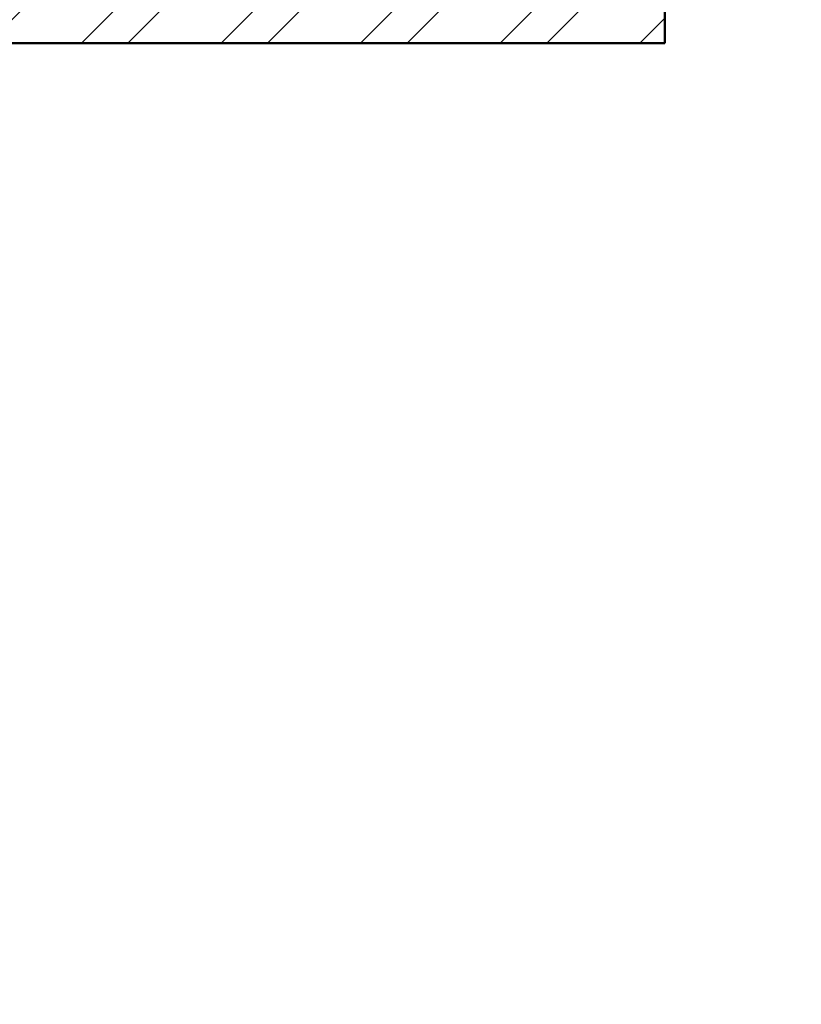
# Model space of a CAD drawing. Units: inches. Extents: x 963 to 2075, y 289 to 2657.
# Tile 66 of 98: x 1266 to 1342, y 2230 to 2325. Entities that reach past the tile are written whole.
import ezdxf

# ---------------------------------------------------------------- set-up
doc = ezdxf.new("R2010")
doc.units = ezdxf.units.IN
doc.layers.add('A-WALL', color=7, linetype='Continuous', lineweight=50)
doc.layers.add('A-WALL-PATT', color=8, linetype='Continuous', lineweight=13)

msp = doc.modelspace()

# ---------------------------------------------------------------- hatches: boundary and pattern name
at = {"layer": 'A-WALL-PATT'}
h = msp.add_hatch(dxfattribs=at)
h.set_pattern_fill('ANSI32', color=256)
h.paths.add_polyline_path([(1296.922, 2558.318), (1203.922, 2558.318), (1203.922, 2493.818), (1191.533, 2493.818), (1191.533, 2489.318), (1211.063, 2489.318), (1211.063, 2492.02), (1211.063, 2493.818), (1208.422, 2493.818), (1208.422, 2553.818), (1292.422, 2553.818), (1292.422, 2538.863), (1296.922, 2538.863)])
h.paths.add_polyline_path([(1442.422, 2558.318), (1349.422, 2558.318), (1349.422, 2538.943), (1353.922, 2538.943), (1353.922, 2553.818), (1437.922, 2553.818), (1437.922, 2493.818), (1434.542, 2493.818), (1434.542, 2489.318), (1448.311, 2489.318), (1448.311, 2491.568), (1448.311, 2493.818), (1442.422, 2493.818)])
h.paths.add_polyline_path([(1415.554, 2491.568), (1415.554, 2493.818), (1340.941, 2493.818), (1340.941, 2489.318), (1371.922, 2489.318), (1371.922, 2378.318), (1367.596, 2378.318), (1367.596, 2373.818), (1371.922, 2373.818), (1371.922, 2355.185), (1376.422, 2355.185), (1376.422, 2489.318), (1415.554, 2489.318)])
h.paths.add_polyline_path([(1304.941, 2491.568), (1304.941, 2493.818), (1296.922, 2493.818), (1296.922, 2514.863), (1292.422, 2514.863), (1292.422, 2493.818), (1232.808, 2493.818), (1232.808, 2489.318), (1256.422, 2489.318), (1256.422, 2327.318), (1253.714, 2327.318), (1253.714, 2322.818), (1328.422, 2322.818), (1328.422, 2331.147), (1323.922, 2331.147), (1323.922, 2327.318), (1260.922, 2327.318), (1260.922, 2373.818), (1323.922, 2373.818), (1323.922, 2357.812), (1328.422, 2357.812), (1328.422, 2373.818), (1346.007, 2373.818), (1346.007, 2376.068), (1346.007, 2378.318), (1260.922, 2378.318), (1260.922, 2489.318), (1304.941, 2489.318)])
h.paths.add_polyline_path([(1226.654, 2327.318), (1124.422, 2327.318), (1124.422, 2347.447), (1119.922, 2347.447), (1119.922, 2322.818), (1163.422, 2322.818), (1163.422, 2305.435), (1165.672, 2305.435), (1167.922, 2305.435), (1167.922, 2322.818), (1226.654, 2322.818), (1226.654, 2325.068)])
h.paths.add_polyline_path([(1095.922, 2489.318), (1124.422, 2489.318), (1131.533, 2489.318), (1131.533, 2491.568), (1131.533, 2493.818), (1119.922, 2493.818), (1091.422, 2493.818), (1091.422, 2417.318), (1095.922, 2417.318), (1119.922, 2417.318), (1119.922, 2407.447), (1124.422, 2407.447), (1124.422, 2421.818), (1095.922, 2421.818)])
h.paths.add_polyline_path([(1512.922, 2558.318), (1508.422, 2558.318), (1508.422, 2493.818), (1503.401, 2493.818), (1503.401, 2489.318), (1508.422, 2489.318), (1508.422, 2327.318), (1376.422, 2327.318), (1376.422, 2330.273), (1371.922, 2330.273), (1371.922, 2298.744), (1376.422, 2298.744), (1376.422, 2322.818), (1508.422, 2322.818), (1508.422, 2165.318), (1504.255, 2165.318), (1504.255, 2160.818), (1508.422, 2160.818), (1508.422, 2108.318), (1512.922, 2108.318), (1512.922, 2160.818), (1516.182, 2160.818), (1516.182, 2163.068), (1516.182, 2165.318), (1512.922, 2165.318), (1512.922, 2322.818), (1644.922, 2322.818), (1644.922, 2298.744), (1649.422, 2298.744), (1649.422, 2322.818), (1649.422, 2330.944), (1647.172, 2330.944), (1644.922, 2330.944), (1644.922, 2327.318), (1512.922, 2327.318), (1512.922, 2489.318), (1516.759, 2489.318), (1516.759, 2491.568), (1516.759, 2493.818), (1512.922, 2493.818)])
h.paths.add_polyline_path([(1671.922, 2558.318), (1578.922, 2558.318), (1578.922, 2493.818), (1573.526, 2493.818), (1573.526, 2489.318), (1586.537, 2489.318), (1586.537, 2491.568), (1586.537, 2493.818), (1583.422, 2493.818), (1583.422, 2553.818), (1667.422, 2553.818), (1667.422, 2541.109), (1671.922, 2541.109)])
h.paths.add_polyline_path([(1681.257, 2493.818), (1671.922, 2493.818), (1671.922, 2517.109), (1667.422, 2517.109), (1667.422, 2493.818), (1610.218, 2493.818), (1610.218, 2489.318), (1644.922, 2489.318), (1644.922, 2357.865), (1649.422, 2357.865), (1649.422, 2373.818), (1652.203, 2373.818), (1652.203, 2375.827), (1652.203, 2378.318), (1649.422, 2378.318), (1649.422, 2489.318), (1681.257, 2489.318), (1681.257, 2491.568)])
h.paths.add_polyline_path([(1821.922, 2558.318), (1728.922, 2558.318), (1728.922, 2541), (1733.422, 2541), (1733.422, 2553.818), (1817.422, 2553.818), (1817.422, 2493.818), (1813.507, 2493.818), (1813.507, 2489.318), (1830.078, 2489.318), (1830.078, 2491.568), (1830.078, 2493.818), (1821.922, 2493.818)])
h.paths.add_polyline_path([(1794.244, 2493.818), (1717.257, 2493.818), (1717.257, 2489.318), (1760.422, 2489.318), (1760.422, 2378.318), (1674.401, 2378.318), (1674.401, 2373.818), (1692.922, 2373.818), (1692.922, 2356.954), (1697.422, 2356.954), (1697.422, 2373.818), (1760.422, 2373.818), (1760.422, 2327.318), (1697.422, 2327.318), (1697.422, 2333.341), (1692.922, 2333.341), (1692.922, 2322.818), (1768.037, 2322.818), (1768.037, 2325.068), (1768.037, 2327.318), (1764.922, 2327.318), (1764.922, 2489.318), (1794.244, 2489.318)])
h.paths.add_polyline_path([(1733.422, 2517), (1728.922, 2517), (1728.922, 2493.818), (1733.422, 2493.818)], flags=17)
h.paths.add_polyline_path([(1929.922, 2493.818), (1890.078, 2493.818), (1890.078, 2489.318), (1896.922, 2489.318), (1925.422, 2489.318), (1925.422, 2421.818), (1896.922, 2421.818), (1896.922, 2408.318), (1901.422, 2408.318), (1901.422, 2417.318), (1925.422, 2417.318), (1929.922, 2417.318)])
h.paths.add_polyline_path([(1901.422, 2348.318), (1896.922, 2348.318), (1896.922, 2327.318), (1800.423, 2327.318), (1800.423, 2322.818), (1853.422, 2322.818), (1853.422, 2309.453), (1857.922, 2309.453), (1857.922, 2322.818), (1901.422, 2322.818)])
h.paths.add_polyline_path([(1857.922, 2249.453), (1853.422, 2249.453), (1853.422, 2214.818), (1686.309, 2214.818), (1686.309, 2210.318), (1853.422, 2210.318), (1853.422, 2202.134), (1857.922, 2202.134), (1857.922, 2210.318)])
h.paths.add_polyline_path([(1857.922, 2142.134), (1853.422, 2142.134), (1853.422, 2115.422), (1841.422, 2115.422), (1841.422, 2088.531), (1841.422, 2046.949), (1845.922, 2046.949), (1845.922, 2110.922), (1905.922, 2110.922), (1905.922, 2092.517), (1910.422, 2092.517), (1910.422, 2115.422), (1857.922, 2115.422)])
h.paths.add_polyline_path([(1532.436, 1482.342), (1573.456, 1482.342), (1573.456, 1501), (1532.436, 1501)], flags=9)
h.paths.add_polyline_path([(1438.658, 1486.302), (1479.678, 1486.302), (1479.678, 1504.96), (1438.658, 1504.96)], flags=9)
h.paths.add_polyline_path([(1411.215, 1365.308), (1659.139, 1365.308), (1659.139, 1402.401), (1411.215, 1402.401)], flags=9)
h.paths.add_polyline_path([(1185.671, 2296.298), (1248.16, 2296.298), (1248.16, 2314.955), (1185.671, 2314.955)], flags=9)
h.paths.add_polyline_path([(1177.31, 2187.35), (1216.15, 2187.35), (1216.15, 2206.007), (1177.31, 2206.007)], flags=9)
h.paths.add_polyline_path([(1295.101, 1602.083), (1328.26, 1602.083), (1328.26, 1620.741), (1295.101, 1620.741)], flags=9)
h.paths.add_polyline_path([(1525.126, 2005.99), (1558.39, 2005.99), (1558.39, 2024.648), (1525.126, 2024.648)], flags=9)
h.paths.add_polyline_path([(1459.606, 1977.125), (1472.195, 1977.125), (1472.195, 1987.429), (1459.606, 1987.429)], flags=9)
h.paths.add_polyline_path([(1467.815, 2053.676), (1480.018, 2053.676), (1480.018, 2063.979), (1467.815, 2063.979)], flags=9)
h.paths.add_polyline_path([(1555.184, 2119.02), (1584.563, 2119.02), (1584.563, 2137.678), (1555.184, 2137.678)], flags=25)
h.paths.add_polyline_path([(1405.389, 2115.291), (1444.478, 2115.291), (1444.478, 2133.948), (1405.389, 2133.948)], flags=25)
h.paths.add_polyline_path([(1698.482, 2004.259), (1727.695, 2004.259), (1727.695, 2022.916), (1698.482, 2022.916)], flags=9)
h.paths.add_polyline_path([(1612.158, 1972.855), (1629.016, 1972.855), (1629.016, 1983.159), (1612.158, 1983.159)], flags=9)
h.paths.add_polyline_path([(1608.289, 2060.036), (1625.147, 2060.036), (1625.147, 2070.34), (1608.289, 2070.34)], flags=9)
h.paths.add_polyline_path([(1527.954, 1684.402), (1566.795, 1684.402), (1566.795, 1703.06), (1527.954, 1703.06)], flags=9)
h.paths.add_polyline_path([(1422.792, 1683.59), (1461.633, 1683.59), (1461.633, 1702.247), (1422.792, 1702.247)], flags=9)
h.paths.add_polyline_path([(1531.262, 1732.459), (1574.015, 1732.459), (1574.015, 1751.116), (1531.262, 1751.116)], flags=9)
h.paths.add_polyline_path([(1402.872, 1732.845), (1439.799, 1732.845), (1439.799, 1751.502), (1402.872, 1751.502)], flags=9)
h.paths.add_polyline_path([(1243.122, 1923.132), (1281.962, 1923.132), (1281.962, 1941.79), (1243.122, 1941.79)], flags=9)
h.paths.add_polyline_path([(1181.752, 1792.268), (1244.241, 1792.268), (1244.241, 1810.926), (1181.752, 1810.926)], flags=9)
h.paths.add_polyline_path([(1265.822, 1670.3), (1316.071, 1670.3), (1316.071, 1688.957), (1265.822, 1688.957)], flags=9)
h.paths.add_polyline_path([(1140.263, 1676.054), (1179.104, 1676.054), (1179.104, 1694.711), (1140.263, 1694.711)], flags=9)
h.paths.add_polyline_path([(1107.49, 1490.889), (1143.374, 1490.889), (1143.374, 1509.546), (1107.49, 1509.546)], flags=9)
h.paths.add_polyline_path([(1217.584, 1483.899), (1246.741, 1483.899), (1246.741, 1502.556), (1217.584, 1502.556)], flags=9)
h.paths.add_polyline_path([(1389.21, 1486.919), (1418.367, 1486.919), (1418.367, 1505.576), (1389.21, 1505.576)], flags=9)
h.paths.add_polyline_path([(1672.208, 1602.083), (1705.366, 1602.083), (1705.366, 1620.741), (1672.208, 1620.741)], flags=9)
h.paths.add_polyline_path([(1752.082, 1522.638), (1781.24, 1522.638), (1781.24, 1541.295), (1752.082, 1541.295)], flags=9)
h.paths.add_polyline_path([(1848.275, 1491.26), (1884.158, 1491.26), (1884.158, 1509.918), (1848.275, 1509.918)], flags=9)
h.paths.add_polyline_path([(1822.47, 1685.62), (1861.31, 1685.62), (1861.31, 1704.278), (1822.47, 1704.278)], flags=9)
h.paths.add_polyline_path([(1713.195, 1672.232), (1763.444, 1672.232), (1763.444, 1690.889), (1713.195, 1690.889)], flags=9)
h.paths.add_polyline_path([(1736.619, 1790.578), (1799.109, 1790.578), (1799.109, 1809.235), (1736.619, 1809.235)], flags=9)
h.paths.add_polyline_path([(1691.491, 1916.355), (1730.332, 1916.355), (1730.332, 1935.013), (1691.491, 1935.013)], flags=9)
h.paths.add_polyline_path([(1764.872, 1973.922), (1794.306, 1973.922), (1794.306, 1992.58), (1764.872, 1992.58)], flags=9)
h.paths.add_polyline_path([(1767.854, 2034.017), (1797.288, 2034.017), (1797.288, 2052.674), (1767.854, 2052.674)], flags=9)
h.paths.add_polyline_path([(1851.593, 2060.331), (1880.751, 2060.331), (1880.751, 2078.989), (1851.593, 2078.989)], flags=25)
h.paths.add_polyline_path([(1688.491, 2086.874), (1727.332, 2086.874), (1727.332, 2105.531), (1688.491, 2105.531)], flags=9)
h.paths.add_polyline_path([(1537.743, 2293.581), (1580.495, 2293.581), (1580.495, 2312.239), (1537.743, 2312.239)], flags=25)
h.paths.add_polyline_path([(1425.587, 2296.109), (1468.34, 2296.109), (1468.34, 2314.766), (1425.587, 2314.766)], flags=25)
h.paths.add_polyline_path([(1278.518, 2004.184), (1307.72, 2004.184), (1307.72, 2022.841), (1278.518, 2022.841)], flags=9)
h.paths.add_polyline_path([(1193.282, 1973.635), (1222.715, 1973.635), (1222.715, 1992.292), (1193.282, 1992.292)], flags=9)
h.paths.add_polyline_path([(1192.411, 2040.577), (1221.845, 2040.577), (1221.845, 2059.234), (1192.411, 2059.234)], flags=9)
h.paths.add_polyline_path([(1130.603, 1951.393), (1159.76, 1951.393), (1159.76, 1970.05), (1130.603, 1970.05)], flags=9)
h.paths.add_polyline_path([(1132.827, 2052.494), (1161.984, 2052.494), (1161.984, 2071.151), (1132.827, 2071.151)], flags=9)
h.paths.add_polyline_path([(1265.128, 2334.619), (1315.377, 2334.619), (1315.377, 2353.277), (1265.128, 2353.277)], flags=25)
h.paths.add_polyline_path([(1136.741, 2330.785), (1175.582, 2330.785), (1175.582, 2349.443), (1136.741, 2349.443)], flags=9)
h.paths.add_polyline_path([(1287.422, 2417.204), (1320.58, 2417.204), (1320.58, 2435.861), (1287.422, 2435.861)], flags=25)
h.paths.add_polyline_path([(1430.988, 2329.159), (1469.828, 2329.159), (1469.828, 2347.816), (1430.988, 2347.816)], flags=25)
h.paths.add_polyline_path([(1525.424, 2329.213), (1564.264, 2329.213), (1564.264, 2347.87), (1525.424, 2347.87)], flags=25)
h.paths.add_polyline_path([(1684.525, 2382.799), (1717.683, 2382.799), (1717.683, 2401.457), (1684.525, 2401.457)], flags=25)
h.paths.add_polyline_path([(1704.805, 2340.293), (1755.054, 2340.293), (1755.054, 2358.95), (1704.805, 2358.95)], flags=25)
h.paths.add_polyline_path([(1694.113, 2287.757), (1756.602, 2287.757), (1756.602, 2306.414), (1694.113, 2306.414)], flags=9)
h.paths.add_polyline_path([(1815.778, 2329.861), (1854.618, 2329.861), (1854.618, 2348.518), (1815.778, 2348.518)], flags=9)
h.paths.add_polyline_path([(1842.873, 2514.256), (1878.756, 2514.256), (1878.756, 2532.914), (1842.873, 2532.914)], flags=9)
h.paths.add_polyline_path([(1769.513, 2531.447), (1798.671, 2531.447), (1798.671, 2550.104), (1769.513, 2550.104)], flags=25)
h.paths.add_polyline_path([(1594.772, 2518.468), (1623.93, 2518.468), (1623.93, 2537.125), (1594.772, 2537.125)], flags=25)
h.paths.add_polyline_path([(1520.723, 2516.185), (1556.606, 2516.185), (1556.606, 2534.842), (1520.723, 2534.842)], flags=25)
h.paths.add_polyline_path([(1464.456, 2516.694), (1500.34, 2516.694), (1500.34, 2535.351), (1464.456, 2535.351)], flags=25)
h.paths.add_polyline_path([(1365.696, 2528.97), (1394.854, 2528.97), (1394.854, 2547.627), (1365.696, 2547.627)], flags=25)
h.paths.add_polyline_path([(1222.838, 2516.231), (1251.995, 2516.231), (1251.995, 2534.889), (1222.838, 2534.889)], flags=25)
h.paths.add_polyline_path([(1104.545, 2509.6), (1140.429, 2509.6), (1140.429, 2528.257), (1104.545, 2528.257)], flags=9)

# ---------------------------------------------------------------- linework, layer by layer
at = {"layer": 'A-WALL'}
for p in [(1328.422, 2331.147), (1253.714, 2322.818)]:
    msp.add_line(p, (1328.422, 2322.818), dxfattribs=at)

doc.saveas('drawing.dxf')
